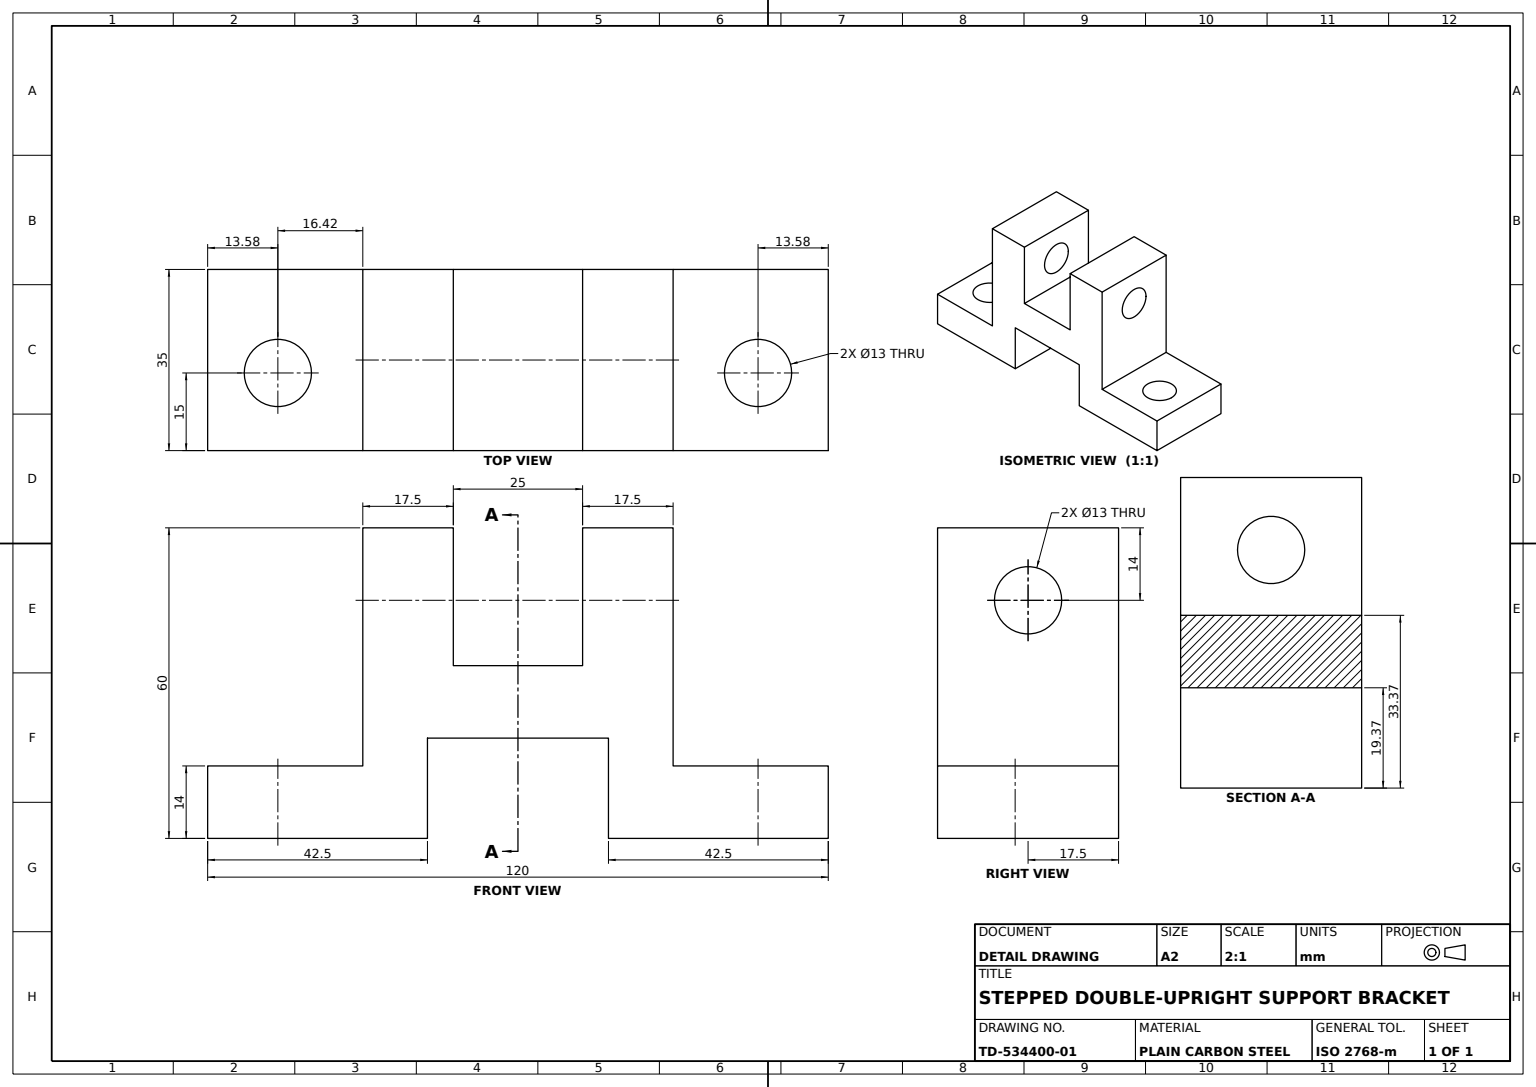
from build123d import *

# Parameters (mm, degrees)
FORK_BODY_DEPTH                 = 35
LUG_CROSS_HOLE_SKETCH_R         = 6.5
LUG_CROSS_HOLE_13_DEPTH         = 105.763638969
BASE_MOUNTING_HOLES_SKETCH_R    = 6.5
BASE_MOUNTING_HOLES_2X_13_DEPTH = 84.312664103


with BuildPart() as part:
    # Fork Profile Sketch → Fork Body (new body)
    with BuildSketch(Plane.XY):
        Polygon((0, 0), (17.5, 0), (17.5, -19.374637846), (60, -19.374637846), (60, -5.374637846), (30, -5.374637846), (30, 40.625362154), (12.5, 40.625362154), (12.5, 14), (-12.5, 14), (-12.5, 40.625362154), (-30, 40.625362154), (-30, -5.374637846), (-60, -5.374637846), (-60, -19.374637846), (-17.5, -19.374637846), (-17.5, 0), align=None)
    extrude(amount=FORK_BODY_DEPTH)

    # Lug Cross Hole Sketch → Lug Cross Hole Ø13 (cut, through all)
    with BuildSketch(Plane.ZY.offset(30)):
        with Locations((17.5, 26.625362154)):
            Circle(LUG_CROSS_HOLE_SKETCH_R)
    extrude(amount=-LUG_CROSS_HOLE_13_DEPTH, mode=Mode.SUBTRACT)

    # Base Mounting Holes Sketch → Base Mounting Holes 2xØ13 (cut, through all)
    with BuildSketch(Plane(origin=(0, -5.374637846, 0), x_dir=(1, 0, 0), z_dir=(0, 1, 0))):
        with Locations(Location((46.423898933, -20, 0), (0, 0, 180))):
            Circle(BASE_MOUNTING_HOLES_SKETCH_R)
        with Locations((-46.423898933, -20)):
            Circle(BASE_MOUNTING_HOLES_SKETCH_R)
    extrude(amount=-BASE_MOUNTING_HOLES_2X_13_DEPTH, mode=Mode.SUBTRACT)


solid = part.part
